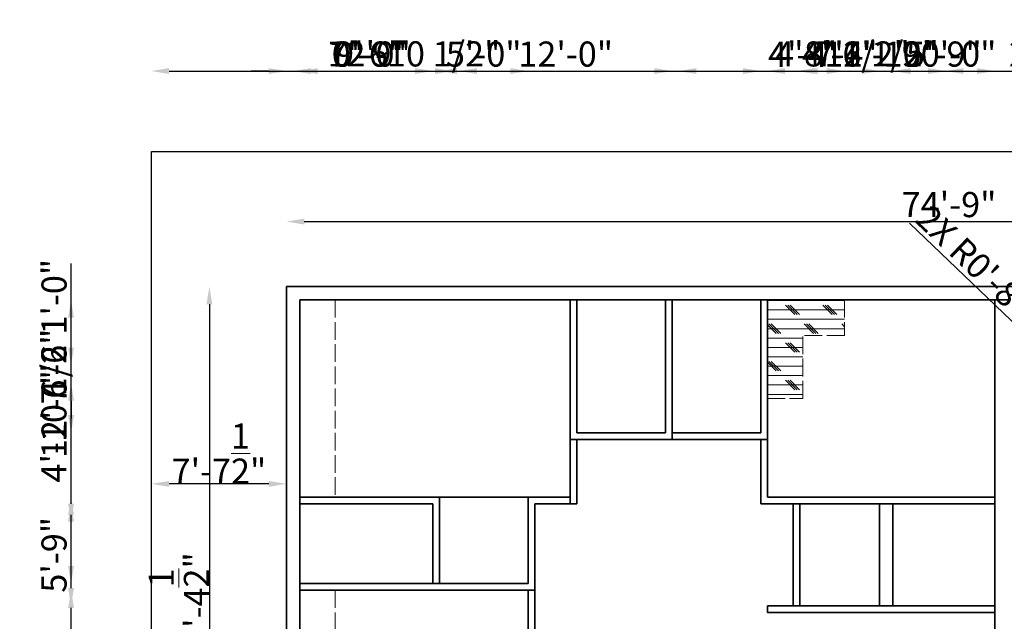
# Model space of a CAD drawing. Units: millimetres. Extents: x 1980 to 3220, y 1535 to 2343.
# Tile 2 of 3: x 1980 to 2647, y 1936 to 2343. Entities that reach past the tile are written whole.
import ezdxf

# ---------------------------------------------------------------- set-up
doc = ezdxf.new("R2010")
doc.units = ezdxf.units.MM
doc.linetypes.add('ACAD_ISO02W100', pattern=[15, 12, -3])
for name, color, linetype, lineweight in [('A-ANNO-DIMS', 2, 'Continuous', 18), ('A-FLOR-FIXT', 9, 'Continuous', 18), ('A-FLOR-FIXT-OVHD', 9, 'ACAD_ISO02W100', 18), ('A-FLOR-FIXT-PATT', 252, 'ACAD_ISO02W100', 13), ('A-WALL', 7, 'Continuous', 35), ('C-PROP', 8, 'Continuous', 25)]:
    doc.layers.add(name, color=color, linetype=linetype, lineweight=lineweight)
doc.styles.get("Standard").update_dxf_attribs({"font": 'arial.ttf'})
doc.dimstyles.new('ISO-25', dxfattribs={"dimtxt": 17, "dimasz": 12, "dimexe": 1.25, "dimexo": 0.625, "dimtad": 1, "dimdec": 1, "dimlunit": 4, "dimtxsty": 'Standard', "dimcen": 2.5, "dimse1": 1, "dimse2": 1, "dimadec": 0, "dimazin": 0, "dimtfac": 1, "dimtdec": 1, "dimtmove": 0, "dimatfit": 3, "dimfxl": 1, "dimarcsym": 0})

# ---------------------------------------------------------------- blocks, each defined once
blk = doc.blocks.new('*D1')
at = {"layer": 'A-ANNO-DIMS', "color": 0, "lineweight": -2, "transparency": 16777216}
blk.add_line((2173.01, 2206.08), (3046.01, 2206.08), dxfattribs=at)
at = {"layer": 'A-ANNO-DIMS', "color": 0, "transparency": 16777216}
for points in [[(2173.01, 2208.08), (2173.01, 2204.08), (2161.01, 2206.08)], [(3046.01, 2208.08), (3046.01, 2204.08), (3058.01, 2206.08)]]:
    blk.add_solid(points, dxfattribs=at)
at = {"layer": 'Defpoints', "color": 0, "transparency": 16777216}
for p in [(3058.01, 2206.08), (2161.01, 2162.1), (3058.01, 2162.1)]:
    blk.add_point(p, dxfattribs=at)
at = {"layer": 'A-ANNO-DIMS', "color": 0, "transparency": 16777216, "insert": (2609.51, 2215.39), "char_height": 17, "attachment_point": 5}
blk.add_mtext('74\'-9"', dxfattribs=at)
blk = doc.blocks.new('*D7')
at = {"layer": 'A-ANNO-DIMS', "color": 0, "lineweight": -2, "transparency": 16777216}
blk.add_line((2149.01, 2028.59), (2081.51, 2028.59), dxfattribs=at)
at = {"layer": 'A-ANNO-DIMS', "color": 0, "transparency": 16777216}
for points in [[(2081.51, 2030.59), (2081.51, 2026.59), (2069.51, 2028.59)], [(2149.01, 2030.59), (2149.01, 2026.59), (2161.01, 2028.59)]]:
    blk.add_solid(points, dxfattribs=at)
at = {"layer": 'Defpoints', "color": 0, "transparency": 16777216}
for p in [(2069.51, 2028.59), (2069.51, 2028.59), (2161.01, 2028.59)]:
    blk.add_point(p, dxfattribs=at)
at = {"layer": 'A-ANNO-DIMS', "color": 0, "transparency": 16777216, "insert": (2115.26, 2049.12), "char_height": 17, "attachment_point": 5}
blk.add_mtext('7\'-7{\\H1x;\\S1/2;}"', dxfattribs=at)
blk = doc.blocks.new('*D8')
at = {"layer": 'A-ANNO-DIMS', "color": 0, "lineweight": -2, "transparency": 16777216}
blk.add_line((2108.81, 2150.1), (2108.81, 1737.6), dxfattribs=at)
at = {"layer": 'A-ANNO-DIMS', "color": 0, "transparency": 16777216}
for points in [[(2106.81, 2150.1), (2110.81, 2150.1), (2108.81, 2162.1)], [(2106.81, 1737.6), (2110.81, 1737.6), (2108.81, 1725.6)]]:
    blk.add_solid(points, dxfattribs=at)
at = {"layer": 'Defpoints', "color": 0, "transparency": 16777216}
for p in [(2161.01, 2162.1), (2108.81, 1725.6), (2161.01, 1725.6)]:
    blk.add_point(p, dxfattribs=at)
at = {"layer": 'A-ANNO-DIMS', "color": 0, "transparency": 16777216, "insert": (2088.13, 1943.85), "char_height": 17, "attachment_point": 5, "rotation": 90}
blk.add_mtext('36\'-4{\\H1x;\\S1/2;}"', dxfattribs=at)
blk = doc.blocks.new('*D9')
at = {"layer": 'A-ANNO-DIMS', "color": 0, "lineweight": -2, "transparency": 16777216}
blk.add_line((2081.51, 2307.95), (3137.51, 2307.95), dxfattribs=at)
at = {"layer": 'A-ANNO-DIMS', "color": 0, "transparency": 16777216}
for points in [[(2081.51, 2309.95), (2081.51, 2305.95), (2069.51, 2307.95)], [(3137.51, 2309.95), (3137.51, 2305.95), (3149.51, 2307.95)]]:
    blk.add_solid(points, dxfattribs=at)
at = {"layer": 'Defpoints', "color": 0, "transparency": 16777216}
for p in [(3149.51, 2307.95), (2069.51, 2253.6), (3149.51, 2253.6)]:
    blk.add_point(p, dxfattribs=at)
at = {"layer": 'A-ANNO-DIMS', "color": 0, "transparency": 16777216, "insert": (2609.51, 2317.25), "char_height": 17, "attachment_point": 5}
blk.add_mtext('90\'-0"', dxfattribs=at)
blk = doc.blocks.new('*D11')
at = {"layer": 'A-ANNO-DIMS', "color": 0, "lineweight": -2, "transparency": 16777216}
blk.add_line((2182.01, 1551.25), (2341.01, 1551.25), dxfattribs=at)
at = {"layer": 'A-ANNO-DIMS', "color": 0, "transparency": 16777216}
for points in [[(2182.01, 1553.25), (2182.01, 1549.25), (2170.01, 1551.25)], [(2341.01, 1553.25), (2341.01, 1549.25), (2353.01, 1551.25)]]:
    blk.add_solid(points, dxfattribs=at)
at = {"layer": 'Defpoints', "color": 0, "transparency": 16777216}
for p in [(2170.01, 2153.1), (2353.01, 2153.1), (2353.01, 1551.25)]:
    blk.add_point(p, dxfattribs=at)
at = {"layer": 'A-ANNO-DIMS', "color": 0, "transparency": 16777216, "insert": (2261.51, 1560.56), "char_height": 17, "attachment_point": 5}
blk.add_mtext('15\'-3"', dxfattribs=at)
blk = doc.blocks.new('*D12')
at = {"layer": 'A-ANNO-DIMS', "color": 0, "lineweight": -2, "transparency": 16777216}
blk.add_line((2369.51, 1551.25), (2405.51, 1551.25), dxfattribs=at)
at = {"layer": 'A-ANNO-DIMS', "color": 0, "transparency": 16777216}
for points in [[(2369.51, 1553.25), (2369.51, 1549.25), (2357.51, 1551.25)], [(2405.51, 1553.25), (2405.51, 1549.25), (2417.51, 1551.25)]]:
    blk.add_solid(points, dxfattribs=at)
at = {"layer": 'Defpoints', "color": 0, "transparency": 16777216}
for p in [(2357.51, 2153.1), (2417.51, 2153.1), (2417.51, 1551.25)]:
    blk.add_point(p, dxfattribs=at)
at = {"layer": 'A-ANNO-DIMS', "color": 0, "transparency": 16777216, "insert": (2387.51, 1560.55), "char_height": 17, "attachment_point": 5}
blk.add_mtext('5\'-0"', dxfattribs=at)
blk = doc.blocks.new('*D13')
at = {"layer": 'A-ANNO-DIMS', "color": 0, "lineweight": -2, "transparency": 16777216}
blk.add_line((2434.01, 1551.25), (2470.01, 1551.25), dxfattribs=at)
at = {"layer": 'A-ANNO-DIMS', "color": 0, "transparency": 16777216}
for points in [[(2434.01, 1553.25), (2434.01, 1549.25), (2422.01, 1551.25)], [(2470.01, 1553.25), (2470.01, 1549.25), (2482.01, 1551.25)]]:
    blk.add_solid(points, dxfattribs=at)
at = {"layer": 'Defpoints', "color": 0, "transparency": 16777216}
for p in [(2422.01, 2153.1), (2482.01, 2153.1), (2482.01, 1551.25)]:
    blk.add_point(p, dxfattribs=at)
at = {"layer": 'A-ANNO-DIMS', "color": 0, "transparency": 16777216, "insert": (2452.01, 1560.55), "char_height": 17, "attachment_point": 5}
blk.add_mtext('5\'-0"', dxfattribs=at)
blk = doc.blocks.new('*D14')
at = {"layer": 'A-ANNO-DIMS', "color": 0, "lineweight": -2, "transparency": 16777216}
blk.add_line((2498.51, 2307.95), (2628.51, 2307.95), dxfattribs=at)
at = {"layer": 'A-ANNO-DIMS', "color": 0, "transparency": 16777216}
for points in [[(2498.51, 2309.95), (2498.51, 2305.95), (2486.51, 2307.95)], [(2628.51, 2309.95), (2628.51, 2305.95), (2640.51, 2307.95)]]:
    blk.add_solid(points, dxfattribs=at)
at = {"layer": 'Defpoints', "color": 0, "transparency": 16777216}
for p in [(2640.51, 2307.95), (2486.51, 2019.6), (2640.51, 2019.6)]:
    blk.add_point(p, dxfattribs=at)
at = {"layer": 'A-ANNO-DIMS', "color": 0, "transparency": 16777216, "insert": (2563.51, 2317.25), "char_height": 17, "attachment_point": 5}
blk.add_mtext('12\'-10"', dxfattribs=at)
blk = doc.blocks.new('*D15')
at = {"layer": 'A-ANNO-DIMS', "color": 0, "lineweight": -2, "transparency": 16777216}
blk.add_line((3203.86, 2031.6), (3203.86, 2141.1), dxfattribs=at)
at = {"layer": 'A-ANNO-DIMS', "color": 0, "transparency": 16777216}
for points in [[(3201.86, 2141.1), (3205.86, 2141.1), (3203.86, 2153.1)], [(3201.86, 2031.6), (3205.86, 2031.6), (3203.86, 2019.6)]]:
    blk.add_solid(points, dxfattribs=at)
at = {"layer": 'Defpoints', "color": 0, "transparency": 16777216}
for p in [(2170.01, 2153.1), (3203.86, 2153.1), (2170.01, 2019.6)]:
    blk.add_point(p, dxfattribs=at)
at = {"layer": 'A-ANNO-DIMS', "color": 0, "transparency": 16777216, "insert": (3194.44, 2086.35), "char_height": 17, "attachment_point": 5, "rotation": 90}
blk.add_mtext('11\'-1 1/2"', dxfattribs=at)
blk = doc.blocks.new('*D16')
at = {"layer": 'A-ANNO-DIMS', "color": 0, "lineweight": -2, "transparency": 16777216}
blk.add_line((3203.86, 2075.1), (3203.86, 2141.1), dxfattribs=at)
at = {"layer": 'A-ANNO-DIMS', "color": 0, "transparency": 16777216}
for points in [[(3201.86, 2141.1), (3205.86, 2141.1), (3203.86, 2153.1)], [(3201.86, 2075.1), (3205.86, 2075.1), (3203.86, 2063.1)]]:
    blk.add_solid(points, dxfattribs=at)
at = {"layer": 'Defpoints', "color": 0, "transparency": 16777216}
for p in [(2357.51, 2153.1), (3203.86, 2153.1), (2357.51, 2063.1)]:
    blk.add_point(p, dxfattribs=at)
at = {"layer": 'A-ANNO-DIMS', "color": 0, "transparency": 16777216, "insert": (3194.55, 2108.1), "char_height": 17, "attachment_point": 5, "rotation": 90}
blk.add_mtext('7\'-6"', dxfattribs=at)
blk = doc.blocks.new('*D17')
at = {"layer": 'A-ANNO-DIMS', "color": 0, "lineweight": -2, "transparency": 16777216}
blk.add_line((2182.01, 2307.95), (2312.51, 2307.95), dxfattribs=at)
at = {"layer": 'A-ANNO-DIMS', "color": 0, "transparency": 16777216}
for points in [[(2182.01, 2309.95), (2182.01, 2305.95), (2170.01, 2307.95)], [(2312.51, 2309.95), (2312.51, 2305.95), (2324.51, 2307.95)]]:
    blk.add_solid(points, dxfattribs=at)
at = {"layer": 'Defpoints', "color": 0, "transparency": 16777216}
for p in [(2324.51, 2307.95), (2170.01, 1830.6), (2324.51, 1830.6)]:
    blk.add_point(p, dxfattribs=at)
at = {"layer": 'A-ANNO-DIMS', "color": 0, "transparency": 16777216, "insert": (2247.26, 2317.36), "char_height": 17, "attachment_point": 5}
blk.add_mtext('12\'-10 1/2"', dxfattribs=at)
blk = doc.blocks.new('*D18')
at = {"layer": 'A-ANNO-DIMS', "color": 0, "lineweight": -2, "transparency": 16777216}
blk.add_line((2015.16, 1842.6), (2015.16, 1944.6), dxfattribs=at)
at = {"layer": 'A-ANNO-DIMS', "color": 0, "transparency": 16777216}
for points in [[(2013.16, 1944.6), (2017.16, 1944.6), (2015.16, 1956.6)], [(2013.16, 1842.6), (2017.16, 1842.6), (2015.16, 1830.6)]]:
    blk.add_solid(points, dxfattribs=at)
at = {"layer": 'Defpoints', "color": 0, "transparency": 16777216}
for p in [(2015.16, 1956.6), (2324.51, 1956.6), (2324.51, 1830.6)]:
    blk.add_point(p, dxfattribs=at)
at = {"layer": 'A-ANNO-DIMS', "color": 0, "transparency": 16777216, "insert": (2005.85, 1893.6), "char_height": 17, "attachment_point": 5, "rotation": 90}
blk.add_mtext('10\'-6"', dxfattribs=at)
blk = doc.blocks.new('*D19')
at = {"layer": 'A-ANNO-DIMS', "color": 0, "lineweight": -2, "transparency": 16777216}
blk.add_line((2182.01, 2307.95), (2248.01, 2307.95), dxfattribs=at)
at = {"layer": 'A-ANNO-DIMS', "color": 0, "transparency": 16777216}
for points in [[(2182.01, 2309.95), (2182.01, 2305.95), (2170.01, 2307.95)], [(2248.01, 2309.95), (2248.01, 2305.95), (2260.01, 2307.95)]]:
    blk.add_solid(points, dxfattribs=at)
at = {"layer": 'Defpoints', "color": 0, "transparency": 16777216}
for p in [(2260.01, 2307.95), (2170.01, 1961.1), (2260.01, 1961.1)]:
    blk.add_point(p, dxfattribs=at)
at = {"layer": 'A-ANNO-DIMS', "color": 0, "transparency": 16777216, "insert": (2215.01, 2317.25), "char_height": 17, "attachment_point": 5}
blk.add_mtext('7\'-6"', dxfattribs=at)
blk = doc.blocks.new('*D20')
at = {"layer": 'A-ANNO-DIMS', "color": 0, "lineweight": -2, "transparency": 16777216}
blk.add_line((2276.51, 2307.95), (2312.51, 2307.95), dxfattribs=at)
at = {"layer": 'A-ANNO-DIMS', "color": 0, "transparency": 16777216}
for points in [[(2276.51, 2309.95), (2276.51, 2305.95), (2264.51, 2307.95)], [(2312.51, 2309.95), (2312.51, 2305.95), (2324.51, 2307.95)]]:
    blk.add_solid(points, dxfattribs=at)
at = {"layer": 'Defpoints', "color": 0, "transparency": 16777216}
for p in [(2324.51, 2307.95), (2264.51, 1961.1), (2324.51, 1961.1)]:
    blk.add_point(p, dxfattribs=at)
at = {"layer": 'A-ANNO-DIMS', "color": 0, "transparency": 16777216, "insert": (2294.51, 2317.25), "char_height": 17, "attachment_point": 5}
blk.add_mtext('5\'-0"', dxfattribs=at)
blk = doc.blocks.new('*D21')
at = {"layer": 'A-ANNO-DIMS', "color": 0, "lineweight": -2, "transparency": 16777216}
for p, q in [((2015.16, 2019.6), (2015.16, 2131.54)), ((2015.16, 1973.1), (2015.16, 2007.6))]:
    blk.add_line(p, q, dxfattribs=at)
at = {"layer": 'A-ANNO-DIMS', "color": 0, "transparency": 16777216}
for points in [[(2013.16, 2007.6), (2017.16, 2007.6), (2015.16, 2019.6)], [(2013.16, 1973.1), (2017.16, 1973.1), (2015.16, 1961.1)]]:
    blk.add_solid(points, dxfattribs=at)
at = {"layer": 'Defpoints', "color": 0, "transparency": 16777216}
for p in [(2015.16, 2019.6), (2324.51, 2019.6), (2324.51, 1961.1)]:
    blk.add_point(p, dxfattribs=at)
at = {"layer": 'A-ANNO-DIMS', "color": 0, "transparency": 16777216, "insert": (2005.74, 2081.57), "char_height": 17, "attachment_point": 5, "rotation": 90}
blk.add_mtext('4\'-10 1/2"', dxfattribs=at)
blk = doc.blocks.new('*D22')
at = {"layer": 'A-ANNO-DIMS', "color": 0, "lineweight": -2, "transparency": 16777216}
blk.add_line((2520.51, 2307.95), (2550.51, 2307.95), dxfattribs=at)
at = {"layer": 'A-ANNO-DIMS', "color": 0, "transparency": 16777216}
for points in [[(2520.51, 2309.95), (2520.51, 2305.95), (2508.51, 2307.95)], [(2550.51, 2309.95), (2550.51, 2305.95), (2562.51, 2307.95)]]:
    blk.add_solid(points, dxfattribs=at)
at = {"layer": 'Defpoints', "color": 0, "transparency": 16777216}
for p in [(2562.51, 2307.95), (2508.51, 1946.1), (2562.51, 1946.1)]:
    blk.add_point(p, dxfattribs=at)
at = {"layer": 'A-ANNO-DIMS', "color": 0, "transparency": 16777216, "insert": (2535.51, 2317.25), "char_height": 17, "attachment_point": 5}
blk.add_mtext('4\'-6"', dxfattribs=at)
blk = doc.blocks.new('*D23')
at = {"layer": 'A-ANNO-DIMS', "color": 0, "lineweight": -2, "transparency": 16777216}
blk.add_line((2583.51, 2307.95), (2628.51, 2307.95), dxfattribs=at)
at = {"layer": 'A-ANNO-DIMS', "color": 0, "transparency": 16777216}
for points in [[(2583.51, 2309.95), (2583.51, 2305.95), (2571.51, 2307.95)], [(2628.51, 2309.95), (2628.51, 2305.95), (2640.51, 2307.95)]]:
    blk.add_solid(points, dxfattribs=at)
at = {"layer": 'Defpoints', "color": 0, "transparency": 16777216}
for p in [(2640.51, 2307.95), (2571.51, 1946.1), (2640.51, 1946.1)]:
    blk.add_point(p, dxfattribs=at)
at = {"layer": 'A-ANNO-DIMS', "color": 0, "transparency": 16777216, "insert": (2606.01, 2317.25), "char_height": 17, "attachment_point": 5}
blk.add_mtext('5\'-9"', dxfattribs=at)
blk = doc.blocks.new('*D24')
at = {"layer": 'A-ANNO-DIMS', "color": 0, "lineweight": -2, "transparency": 16777216}
blk.add_line((2015.16, 1958.1), (2015.16, 2003.1), dxfattribs=at)
at = {"layer": 'A-ANNO-DIMS', "color": 0, "transparency": 16777216}
for points in [[(2013.16, 2003.1), (2017.16, 2003.1), (2015.16, 2015.1)], [(2013.16, 1958.1), (2017.16, 1958.1), (2015.16, 1946.1)]]:
    blk.add_solid(points, dxfattribs=at)
at = {"layer": 'Defpoints', "color": 0, "transparency": 16777216}
for p in [(2015.16, 2015.1), (2640.51, 2015.1), (2640.51, 1946.1)]:
    blk.add_point(p, dxfattribs=at)
at = {"layer": 'A-ANNO-DIMS', "color": 0, "transparency": 16777216, "insert": (2005.85, 1980.6), "char_height": 17, "attachment_point": 5, "rotation": 90}
blk.add_mtext('5\'-9"', dxfattribs=at)
blk = doc.blocks.new('*D25')
at = {"layer": 'A-ANNO-DIMS', "color": 0, "lineweight": -2, "transparency": 16777216}
blk.add_line((2177.51, 2307.95), (2261.51, 2307.95), dxfattribs=at)
at = {"layer": 'A-ANNO-DIMS', "color": 0, "transparency": 16777216}
for points in [[(2177.51, 2309.95), (2177.51, 2305.95), (2165.51, 2307.95)], [(2261.51, 2309.95), (2261.51, 2305.95), (2273.51, 2307.95)]]:
    blk.add_solid(points, dxfattribs=at)
at = {"layer": 'Defpoints', "color": 0, "transparency": 16777216}
for p in [(2273.51, 2307.95), (2165.51, 1734.6), (2273.51, 1734.6)]:
    blk.add_point(p, dxfattribs=at)
at = {"layer": 'A-ANNO-DIMS', "color": 0, "transparency": 16777216, "insert": (2219.51, 2317.25), "char_height": 17, "attachment_point": 5}
blk.add_mtext('9\'-0"', dxfattribs=at)
blk = doc.blocks.new('*D26')
at = {"layer": 'A-ANNO-DIMS', "color": 0, "lineweight": -2, "transparency": 16777216}
blk.add_line((2290.01, 2307.95), (2410.01, 2307.95), dxfattribs=at)
at = {"layer": 'A-ANNO-DIMS', "color": 0, "transparency": 16777216}
for points in [[(2290.01, 2309.95), (2290.01, 2305.95), (2278.01, 2307.95)], [(2410.01, 2309.95), (2410.01, 2305.95), (2422.01, 2307.95)]]:
    blk.add_solid(points, dxfattribs=at)
at = {"layer": 'Defpoints', "color": 0, "transparency": 16777216}
for p in [(2422.01, 2307.95), (2278.01, 1734.6), (2422.01, 1734.6)]:
    blk.add_point(p, dxfattribs=at)
at = {"layer": 'A-ANNO-DIMS', "color": 0, "transparency": 16777216, "insert": (2350.01, 2317.25), "char_height": 17, "attachment_point": 5}
blk.add_mtext('12\'-0"', dxfattribs=at)
blk = doc.blocks.new('*D29')
at = {"layer": 'A-ANNO-DIMS', "color": 0, "lineweight": -2, "transparency": 16777216}
blk.add_line((2518.6, 2307.95), (2595.26, 2307.95), dxfattribs=at)
at = {"layer": 'A-ANNO-DIMS', "color": 0, "transparency": 16777216}
for points in [[(2518.6, 2309.95), (2518.6, 2305.95), (2506.6, 2307.95)], [(2595.26, 2309.95), (2595.26, 2305.95), (2607.26, 2307.95)]]:
    blk.add_solid(points, dxfattribs=at)
at = {"layer": 'Defpoints', "color": 0, "transparency": 16777216}
for p in [(2607.26, 2307.95), (2506.6, 1734.6), (2607.26, 1734.6)]:
    blk.add_point(p, dxfattribs=at)
at = {"layer": 'A-ANNO-DIMS', "color": 0, "transparency": 16777216, "insert": (2556.93, 2317.36), "char_height": 17, "attachment_point": 5}
blk.add_mtext('8\'-4 1/2"', dxfattribs=at)
blk = doc.blocks.new('*D30')
at = {"layer": 'A-ANNO-DIMS', "color": 0, "lineweight": -2, "transparency": 16777216}
for p, q in [((2619.26, 2307.95), (2628.51, 2307.95)), ((2640.51, 2307.95), (2738.85, 2307.95))]:
    blk.add_line(p, q, dxfattribs=at)
at = {"layer": 'A-ANNO-DIMS', "color": 0, "transparency": 16777216}
for points in [[(2619.26, 2309.95), (2619.26, 2305.95), (2607.26, 2307.95)], [(2628.51, 2309.95), (2628.51, 2305.95), (2640.51, 2307.95)]]:
    blk.add_solid(points, dxfattribs=at)
at = {"layer": 'Defpoints', "color": 0, "transparency": 16777216}
for p in [(2640.51, 2307.95), (2607.26, 1734.6), (2640.51, 1734.6)]:
    blk.add_point(p, dxfattribs=at)
at = {"layer": 'A-ANNO-DIMS', "color": 0, "transparency": 16777216, "insert": (2695.68, 2317.36), "char_height": 17, "attachment_point": 5}
blk.add_mtext('2\'-9 1/2"', dxfattribs=at)
blk = doc.blocks.new('*D34')
at = {"layer": 'A-ANNO-DIMS', "color": 0, "lineweight": -2, "transparency": 16777216}
blk.add_line((2015.16, 2015.1), (2015.16, 2141.1), dxfattribs=at)
at = {"layer": 'A-ANNO-DIMS', "color": 0, "transparency": 16777216}
for points in [[(2013.16, 2141.1), (2017.16, 2141.1), (2015.16, 2153.1)], [(2013.16, 2015.1), (2017.16, 2015.1), (2015.16, 2003.1)]]:
    blk.add_solid(points, dxfattribs=at)
at = {"layer": 'Defpoints', "color": 0, "transparency": 16777216}
for p in [(2015.16, 2153.1), (3049.01, 2153.1), (3049.01, 2003.1)]:
    blk.add_point(p, dxfattribs=at)
at = {"layer": 'A-ANNO-DIMS', "color": 0, "transparency": 16777216, "insert": (2005.85, 2078.1), "char_height": 17, "attachment_point": 5, "rotation": 90}
blk.add_mtext('12\'-6"', dxfattribs=at)
blk = doc.blocks.new('*D35')
at = {"layer": 'A-ANNO-DIMS', "color": 0, "lineweight": -2, "transparency": 16777216}
blk.add_line((2015.16, 2075.1), (2015.16, 2141.1), dxfattribs=at)
at = {"layer": 'A-ANNO-DIMS', "color": 0, "transparency": 16777216}
for points in [[(2013.16, 2141.1), (2017.16, 2141.1), (2015.16, 2153.1)], [(2013.16, 2075.1), (2017.16, 2075.1), (2015.16, 2063.1)]]:
    blk.add_solid(points, dxfattribs=at)
at = {"layer": 'Defpoints', "color": 0, "transparency": 16777216}
for p in [(2015.16, 2153.1), (2923.51, 2153.1), (2923.51, 2063.1)]:
    blk.add_point(p, dxfattribs=at)
at = {"layer": 'A-ANNO-DIMS', "color": 0, "transparency": 16777216, "insert": (2005.85, 2108.1), "char_height": 17, "attachment_point": 5, "rotation": 90}
blk.add_mtext('7\'-6"', dxfattribs=at)
blk = doc.blocks.new('*D48')
at = {"layer": 'A-ANNO-DIMS', "color": 0, "lineweight": -2, "transparency": 16777216}
for p, q in [((2015.16, 2120.82), (2015.16, 2177.66)), ((2015.16, 2096.82), (2015.16, 2108.82)), ((2015.16, 2084.82), (2015.16, 2072.82))]:
    blk.add_line(p, q, dxfattribs=at)
at = {"layer": 'A-ANNO-DIMS', "color": 0, "transparency": 16777216}
for points in [[(2013.16, 2120.82), (2017.16, 2120.82), (2015.16, 2108.82)], [(2013.16, 2084.82), (2017.16, 2084.82), (2015.16, 2096.82)]]:
    blk.add_solid(points, dxfattribs=at)
at = {"layer": 'Defpoints', "color": 0, "transparency": 16777216}
for p in [(2015.16, 2108.82), (2649.51, 2108.82), (2649.51, 2096.82)]:
    blk.add_point(p, dxfattribs=at)
at = {"layer": 'A-ANNO-DIMS', "color": 0, "transparency": 16777216, "insert": (2005.85, 2155.24), "char_height": 17, "attachment_point": 5, "rotation": 90}
blk.add_mtext('1\'-0"', dxfattribs=at)
blk = doc.blocks.new('*D49')
at = {"layer": 'A-ANNO-DIMS', "color": 0, "lineweight": -2, "transparency": 16777216}
for p, q in [((2149.01, 2307.95), (2137.01, 2307.95)), ((2161.01, 2307.95), (2170.01, 2307.95)), ((2182.01, 2307.95), (2240.45, 2307.95))]:
    blk.add_line(p, q, dxfattribs=at)
at = {"layer": 'A-ANNO-DIMS', "color": 0, "transparency": 16777216}
for points in [[(2149.01, 2309.95), (2149.01, 2305.95), (2161.01, 2307.95)], [(2182.01, 2309.95), (2182.01, 2305.95), (2170.01, 2307.95)]]:
    blk.add_solid(points, dxfattribs=at)
at = {"layer": 'Defpoints', "color": 0, "transparency": 16777216}
for p in [(2170.01, 2307.95), (2161.01, 2162.1), (2170.01, 2153.1)]:
    blk.add_point(p, dxfattribs=at)
at = {"layer": 'A-ANNO-DIMS', "color": 0, "transparency": 16777216, "insert": (2217.23, 2317.25), "char_height": 17, "attachment_point": 5}
blk.add_mtext('0\'-9"', dxfattribs=at)
blk = doc.blocks.new('*D50')
at = {"layer": 'A-ANNO-DIMS', "color": 0, "lineweight": -2, "transparency": 16777216}
for p, q in [((2405.51, 1551.25), (2393.51, 1551.25)), ((2417.51, 1551.25), (2422.01, 1551.25)), ((2434.01, 1551.25), (2532.06, 1551.25))]:
    blk.add_line(p, q, dxfattribs=at)
at = {"layer": 'A-ANNO-DIMS', "color": 0, "transparency": 16777216}
for points in [[(2405.51, 1553.25), (2405.51, 1549.25), (2417.51, 1551.25)], [(2434.01, 1553.25), (2434.01, 1549.25), (2422.01, 1551.25)]]:
    blk.add_solid(points, dxfattribs=at)
at = {"layer": 'Defpoints', "color": 0, "transparency": 16777216}
for p in [(2417.51, 2063.1), (2422.01, 2063.1), (2422.01, 1551.25)]:
    blk.add_point(p, dxfattribs=at)
at = {"layer": 'A-ANNO-DIMS', "color": 0, "transparency": 16777216, "insert": (2489.03, 1560.66), "char_height": 17, "attachment_point": 5}
blk.add_mtext('0\'-4 1/2"', dxfattribs=at)
blk = doc.blocks.new('*D51')
at = {"layer": 'A-ANNO-DIMS', "color": 0, "lineweight": -2, "transparency": 16777216}
blk.add_line((2498.508481, 2307.945639), (2526.687065, 2307.945639), dxfattribs=at)
at = {"layer": 'A-ANNO-DIMS', "color": 0, "transparency": 16777216}
for points in [[(2498.508481, 2309.945639), (2498.508481, 2305.945639), (2486.508481, 2307.945639)], [(2526.687065, 2309.945639), (2526.687065, 2305.945639), (2538.687065, 2307.945639)]]:
    blk.add_solid(points, dxfattribs=at)
at = {"layer": 'Defpoints', "color": 0, "transparency": 16777216}
for p in [(2538.687065, 2307.945639), (2486.508481, 2153.095639), (2538.687065, 2153.095639)]:
    blk.add_point(p, dxfattribs=at)
at = {"layer": 'A-ANNO-DIMS', "color": 0, "transparency": 16777216, "insert": (2512.597773, 2317.070639), "char_height": 17, "attachment_point": 5}
blk.add_mtext('4\'-4"', dxfattribs=at)
blk = doc.blocks.new('*D52')
at = {"layer": 'A-ANNO-DIMS', "color": 0, "lineweight": -2, "transparency": 16777216}
blk.add_line((3203.86, 2098.35), (3203.86, 2141.1), dxfattribs=at)
at = {"layer": 'A-ANNO-DIMS', "color": 0, "transparency": 16777216}
for points in [[(3201.86, 2141.1), (3205.86, 2141.1), (3203.86, 2153.1)], [(3201.86, 2098.35), (3205.86, 2098.35), (3203.86, 2086.35)]]:
    blk.add_solid(points, dxfattribs=at)
at = {"layer": 'Defpoints', "color": 0, "transparency": 16777216}
for p in [(2538.69, 2153.1), (3203.86, 2153.1), (2510.51, 2086.35)]:
    blk.add_point(p, dxfattribs=at)
at = {"layer": 'A-ANNO-DIMS', "color": 0, "transparency": 16777216, "insert": (3194.59, 2119.72), "char_height": 17, "attachment_point": 5, "rotation": 90}
blk.add_mtext('5\'-7"', dxfattribs=at)
blk = doc.blocks.new('*D53')
at = {"layer": 'A-ANNO-DIMS', "color": 0, "lineweight": -2, "transparency": 16777216}
for p, q in [((2474.51, 1551.25), (2462.51, 1551.25)), ((2486.51, 1551.25), (2510.51, 1551.25)), ((2522.51, 1551.25), (2581.24, 1551.25))]:
    blk.add_line(p, q, dxfattribs=at)
at = {"layer": 'A-ANNO-DIMS', "color": 0, "transparency": 16777216}
for points in [[(2474.51, 1553.25), (2474.51, 1549.25), (2486.51, 1551.25)], [(2522.51, 1553.25), (2522.51, 1549.25), (2510.51, 1551.25)]]:
    blk.add_solid(points, dxfattribs=at)
at = {"layer": 'Defpoints', "color": 0, "transparency": 16777216}
for p in [(2486.51, 2086.35), (2510.51, 2086.35), (2510.51, 1551.25)]:
    blk.add_point(p, dxfattribs=at)
at = {"layer": 'A-ANNO-DIMS', "color": 0, "transparency": 16777216, "insert": (2557.87, 1560.55), "char_height": 17, "attachment_point": 5}
blk.add_mtext('2\'-0"', dxfattribs=at)
blk = doc.blocks.new('*D54')
at = {"layer": 'A-ANNO-DIMS', "color": 0, "lineweight": -2, "transparency": 16777216}
for p, q in [((2438.51, 2307.95), (2470.01, 2307.95)), ((2482.01, 2307.95), (2580.75, 2307.95))]:
    blk.add_line(p, q, dxfattribs=at)
at = {"layer": 'A-ANNO-DIMS', "color": 0, "transparency": 16777216}
for points in [[(2438.51, 2309.95), (2438.51, 2305.95), (2426.51, 2307.95)], [(2470.01, 2309.95), (2470.01, 2305.95), (2482.01, 2307.95)]]:
    blk.add_solid(points, dxfattribs=at)
at = {"layer": 'Defpoints', "color": 0, "transparency": 16777216}
for p in [(2482.01, 2307.95), (2426.51, 1799.1), (2482.01, 1799.1)]:
    blk.add_point(p, dxfattribs=at)
at = {"layer": 'A-ANNO-DIMS', "color": 0, "transparency": 16777216, "insert": (2537.38, 2317.36), "char_height": 17, "attachment_point": 5}
blk.add_mtext('4\'-7 1/2"', dxfattribs=at)
blk = doc.blocks.new('*D57')
at = {"layer": 'A-ANNO-DIMS', "color": 0, "lineweight": -2, "transparency": 16777216}
for p, q in [((2550.51, 1551.25), (2538.51, 1551.25)), ((2562.51, 1551.25), (2571.51, 1551.25)), ((2583.51, 1551.25), (2641.95, 1551.25))]:
    blk.add_line(p, q, dxfattribs=at)
at = {"layer": 'A-ANNO-DIMS', "color": 0, "transparency": 16777216}
for points in [[(2550.51, 1553.25), (2550.51, 1549.25), (2562.51, 1551.25)], [(2583.51, 1553.25), (2583.51, 1549.25), (2571.51, 1551.25)]]:
    blk.add_solid(points, dxfattribs=at)
at = {"layer": 'Defpoints', "color": 0, "transparency": 16777216}
for p in [(2562.51, 1946.1), (2571.51, 1946.1), (2571.51, 1551.25)]:
    blk.add_point(p, dxfattribs=at)
at = {"layer": 'A-ANNO-DIMS', "color": 0, "transparency": 16777216, "insert": (2618.73, 1560.55), "char_height": 17, "attachment_point": 5}
blk.add_mtext('0\'-9"', dxfattribs=at)
blk = doc.blocks.new('*D58')
at = {"layer": 'A-ANNO-DIMS', "color": 0, "lineweight": -2, "transparency": 16777216}
for p, q in [((2582.78, 2205.03), (2663.33, 2127.9)), ((2677.78, 2114.07), (2672, 2119.6))]:
    blk.add_line(p, q, dxfattribs=at)
at = {"layer": 'A-ANNO-DIMS', "color": 0, "transparency": 16777216}
blk.add_solid([(2664.72, 2129.34), (2661.95, 2126.45), (2672, 2119.6)], dxfattribs=at)
at = {"layer": 'Defpoints', "color": 0, "transparency": 16777216}
for p in [(2672, 2119.6), (2677.78, 2114.07)]:
    blk.add_point(p, dxfattribs=at)
at = {"layer": 'A-ANNO-DIMS', "color": 0, "transparency": 16777216, "insert": (2625.16, 2177.34), "char_height": 17, "attachment_point": 5, "rotation": 316.24382}
blk.add_mtext('2X R0\'-8"', dxfattribs=at)

msp = doc.modelspace()

# ---------------------------------------------------------------- hatches: boundary and pattern name
at = {"layer": 'A-FLOR-FIXT-PATT'}
h = msp.add_hatch(dxfattribs=at)
h.set_pattern_fill('CORK', color=256, scale=2)
h.set_pattern_definition([(0, (0, 0), (0, 6.35), []), (135, (3.175, -3.175), (-12.70001, -12.70001), [8.98026, -8.98026]), (135, (4.763, -3.175), (-12.70001, -12.70001), [8.98026, -8.98026]), (135, (6.35, -3.175), (-12.70001, -12.70001), [8.98026, -8.98026])])
h.paths.add_polyline_path([(2510.51, 2129.1), (2538.69, 2129.1), (2538.69, 2153.1), (2486.51, 2153.1), (2486.51, 2086.35), (2510.51, 2086.35)])

# ---------------------------------------------------------------- linework, layer by layer
at = {"layer": 'A-FLOR-FIXT'}
for p, q in [((2170.01, 2153.1), (2200.01, 2153.1)), ((2170.01, 2153.1), (2194.01, 2153.1)), ((2486.51, 2153.1), (2532.27, 2153.1))]:
    msp.add_line(p, q, dxfattribs=at)
at = {"layer": 'A-FLOR-FIXT-OVHD'}
for p, q in [((2194.01, 2153.1), (2194.01, 2019.6)), ((2538.69, 2153.1), (2538.69, 2129.1)), ((2538.69, 2129.1), (2510.51, 2129.1)), ((2510.51, 2086.35), (2510.51, 2129.1)), ((2486.51, 2086.35), (2510.51, 2086.35)), ((2194.01, 1956.6), (2194.01, 1830.6))]:
    msp.add_line(p, q, dxfattribs=at)
at = {"layer": 'A-WALL'}
for p, q in [((2161.01, 1725.6), (2161.01, 2162.1)), ((2161.01, 2162.1), (3058.01, 2162.1)), ((2170.01, 1830.6), (2170.01, 2153.1)), ((2170.01, 2153.1), (2649.51, 2153.1)), ((2353.01, 2015.1), (2353.01, 2153.1)), ((2357.51, 2063.1), (2357.51, 2153.1)), ((2417.51, 2063.1), (2417.51, 2153.1)), ((2422.01, 2058.6), (2422.01, 2153.1)), ((2482.01, 2063.1), (2482.01, 2153.1)), ((2486.51, 2019.6), (2486.51, 2153.1)), ((2640.51, 1734.6), (2640.51, 2153.1)), ((2357.51, 2063.1), (2417.51, 2063.1)), ((2422.01, 2063.1), (2482.01, 2063.1)), ((2353.01, 2058.6), (2486.51, 2058.6)), ((2357.51, 2015.1), (2357.51, 2058.6)), ((2482.01, 2015.1), (2482.01, 2058.6)), ((2170.01, 2019.6), (2353.01, 2019.6)), ((2170.01, 2015.1), (2260.01, 2015.1)), ((2260.01, 1961.1), (2260.01, 2015.1)), ((2264.51, 1961.1), (2264.51, 2019.6)), ((2324.51, 1961.1), (2324.51, 2019.6)), ((2329.01, 1956.6), (2329.01, 2015.1)), ((2329.01, 2015.1), (2357.51, 2015.1)), ((2482.01, 2015.1), (2640.51, 2015.1)), ((2486.51, 2019.6), (2640.51, 2019.6)), ((2504.01, 1946.1), (2504.01, 2015.1)), ((2508.51, 1946.1), (2508.51, 2015.1)), ((2562.51, 1946.1), (2562.51, 2015.1)), ((2571.51, 1946.1), (2571.51, 2015.1)), ((2170.01, 1961.1), (2264.51, 1961.1)), ((2264.51, 1961.1), (2324.51, 1961.1)), ((2170.01, 1956.6), (2329.01, 1956.6)), ((2324.51, 1956.6), (2324.51, 1830.6)), ((2329.01, 1956.6), (2329.01, 1826.1)), ((2486.51, 1946.1), (2640.51, 1946.1)), ((2486.51, 1941.6), (2486.51, 1946.1)), ((2486.51, 1941.6), (2640.51, 1941.6))]:
    msp.add_line(p, q, dxfattribs=at)
at = {"layer": 'C-PROP'}
msp.add_lwpolyline([(2069.51, 2253.6), (3149.51, 2253.6), (3149.51, 1605.6), (2069.51, 1605.6)], close=True, dxfattribs=at)

# ---------------------------------------------------------------- dimensions: what is measured, and where the dimension line sits
at = {"layer": 'A-ANNO-DIMS'}
for base, p1, p2, override, picture, middle in [((2324.51, 2307.95), (2170.01, 1830.6), (2324.51, 1830.6), {"dimdec": 1, "dimlfac": 1, "dimrnd": 0, "dimzin": 1, "dimdsep": 46, "dimlunit": 4, "dimfrac": 2}, '*D17', (2247.26, 2317.36)), ((2482.01, 2307.95), (2426.51, 1799.1), (2482.01, 1799.1), {"dimdec": 1, "dimlfac": 1, "dimrnd": 0, "dimzin": 1, "dimdsep": 46, "dimlunit": 4, "dimfrac": 2}, '*D54', (2537.38, 2317.36)), ((2607.26, 2307.95), (2506.6, 1734.6), (2607.26, 1734.6), {"dimdec": 1, "dimlfac": 1, "dimrnd": 0, "dimzin": 1, "dimdsep": 46, "dimlunit": 4, "dimfrac": 2}, '*D29', (2556.93, 2317.36)), ((2640.508481, 2307.945639), (2607.258481, 1734.595639), (2640.508481, 1734.595639), {"dimdec": 1, "dimlfac": 1, "dimrnd": 0, "dimzin": 1, "dimdsep": 46, "dimlunit": 4, "dimfrac": 2}, '*D30', (2695.67986572, 2317.3605435)), ((3149.51, 2307.95), (2069.51, 2253.6), (3149.51, 2253.6), {"dimdec": 1, "dimlfac": 1, "dimrnd": 0, "dimzin": 1, "dimdsep": 46, "dimlunit": 4, "dimfrac": 2}, '*D9', (2609.51, 2317.25)), ((2170.01, 2307.95), (2161.01, 2162.1), (2170.01, 2153.1), {"dimdec": 1, "dimlfac": 1, "dimrnd": 0, "dimzin": 1, "dimdsep": 46, "dimlunit": 4, "dimfrac": 2}, '*D49', (2217.23, 2317.25)), ((2273.51, 2307.95), (2165.51, 1734.6), (2273.51, 1734.6), {"dimdec": 1, "dimlfac": 1, "dimrnd": 0, "dimzin": 1, "dimdsep": 46, "dimlunit": 4, "dimfrac": 2}, '*D25', (2219.51, 2317.25)), ((2260.01, 2307.95), (2170.01, 1961.1), (2260.01, 1961.1), {"dimdec": 1, "dimlfac": 1, "dimrnd": 0, "dimzin": 1, "dimdsep": 46, "dimlunit": 4, "dimfrac": 2}, '*D19', (2215.01, 2317.25)), ((2324.51, 2307.95), (2264.51, 1961.1), (2324.51, 1961.1), {"dimdec": 1, "dimlfac": 1, "dimrnd": 0, "dimzin": 1, "dimdsep": 46, "dimlunit": 4, "dimfrac": 2}, '*D20', (2294.51, 2317.25)), ((2422.01, 2307.95), (2278.01, 1734.6), (2422.01, 1734.6), {"dimdec": 1, "dimlfac": 1, "dimrnd": 0, "dimzin": 1, "dimdsep": 46, "dimlunit": 4, "dimfrac": 2}, '*D26', (2350.01, 2317.25)), ((2640.51, 2307.95), (2486.51, 2019.6), (2640.51, 2019.6), {"dimdec": 1, "dimlfac": 1, "dimrnd": 0, "dimzin": 1, "dimdsep": 46, "dimlunit": 4, "dimfrac": 2}, '*D14', (2563.51, 2317.25)), ((2538.69, 2307.95), (2486.51, 2153.1), (2538.69, 2153.1), {"dimdec": 1, "dimlfac": 1, "dimrnd": 0, "dimzin": 1, "dimdsep": 46, "dimlunit": 4, "dimfrac": 2}, '*D51', (2512.6, 2317.07)), ((2562.51, 2307.95), (2508.51, 1946.1), (2562.51, 1946.1), {"dimdec": 1, "dimlfac": 1, "dimrnd": 0, "dimzin": 1, "dimdsep": 46, "dimlunit": 4, "dimfrac": 2}, '*D22', (2535.51, 2317.25)), ((2640.51, 2307.95), (2571.51, 1946.1), (2640.51, 1946.1), {"dimdec": 1, "dimlfac": 1, "dimrnd": 0, "dimzin": 1, "dimdsep": 46, "dimlunit": 4, "dimfrac": 2}, '*D23', (2606.01, 2317.25)), ((3058.01, 2206.08), (2161.01, 2162.1), (3058.01, 2162.1), {"dimclrd": 0, "dimclre": 0, "dimclrt": 0}, '*D1', (2609.51, 2215.39)), ((2353.01, 1551.25), (2170.01, 2153.1), (2353.01, 2153.1), {"dimdec": 1, "dimlfac": 1, "dimrnd": 0, "dimzin": 1, "dimdsep": 46, "dimlunit": 4, "dimfrac": 2}, '*D11', (2261.51, 1560.56)), ((2417.51, 1551.25), (2357.51, 2153.1), (2417.51, 2153.1), {"dimdec": 1, "dimlfac": 1, "dimrnd": 0, "dimzin": 1, "dimdsep": 46, "dimlunit": 4, "dimfrac": 2}, '*D12', (2387.51, 1560.55)), ((2482.01, 1551.25), (2422.01, 2153.1), (2482.01, 2153.1), {"dimdec": 1, "dimlfac": 1, "dimrnd": 0, "dimzin": 1, "dimdsep": 46, "dimlunit": 4, "dimfrac": 2}, '*D13', (2452.01, 1560.55)), ((2510.51, 1551.25), (2486.51, 2086.35), (2510.51, 2086.35), {"dimdec": 1, "dimlfac": 1, "dimrnd": 0, "dimzin": 1, "dimdsep": 46, "dimlunit": 4, "dimfrac": 2}, '*D53', (2557.87, 1560.55)), ((2069.51, 2028.59), (2161.01, 2028.59), (2069.51, 2028.59), {"dimclrd": 0, "dimclre": 0, "dimclrt": 0}, '*D7', (2115.26, 2049.12)), ((2422.01, 1551.25), (2417.51, 2063.1), (2422.01, 2063.1), {"dimdec": 1, "dimlfac": 1, "dimrnd": 0, "dimzin": 1, "dimdsep": 46, "dimlunit": 4, "dimfrac": 2}, '*D50', (2489.03, 1560.66)), ((2571.51, 1551.25), (2562.51, 1946.1), (2571.51, 1946.1), {"dimdec": 1, "dimlfac": 1, "dimrnd": 0, "dimzin": 1, "dimdsep": 46, "dimlunit": 4, "dimfrac": 2}, '*D57', (2618.73, 1560.55))]:
    dim = msp.add_linear_dim(base=base, p1=p1, p2=p2, dimstyle='ISO-25', override=override, dxfattribs=at)
    dim.commit()
    dim.dimension.update_dxf_attribs({"geometry": picture, "text_midpoint": middle})
dim = msp.add_radius_dim(center=(2677.78, 2114.07), mpoint=(2672, 2119.6), text='2X <>', dimstyle='ISO-25', override={"dimdec": 1, "dimlfac": 1, "dimrnd": 0, "dimzin": 1, "dimdsep": 46, "dimlunit": 4, "dimfrac": 2}, dxfattribs=at)
dim.commit()
dim.dimension.update_dxf_attribs({"geometry": '*D58', "text_midpoint": (2625.16, 2177.34)})
for base, p1, p2, override, picture, middle in [((2015.16, 2108.82), (2649.51, 2096.82), (2649.51, 2108.82), {"dimdec": 1, "dimlfac": 1, "dimrnd": 0, "dimzin": 1, "dimdsep": 46, "dimlunit": 4, "dimfrac": 2}, '*D48', (2005.85, 2155.24)), ((2108.81, 1725.6), (2161.01, 2162.1), (2161.01, 1725.6), {"dimclrd": 0, "dimclre": 0, "dimclrt": 0}, '*D8', (2088.13, 1943.85)), ((2015.16, 2153.1), (3049.01, 2003.1), (3049.01, 2153.1), {"dimdec": 1, "dimlfac": 1, "dimrnd": 0, "dimzin": 1, "dimdsep": 46, "dimlunit": 4, "dimfrac": 2}, '*D34', (2005.85, 2078.1)), ((2015.16, 2153.1), (2923.51, 2063.1), (2923.51, 2153.1), {"dimdec": 1, "dimlfac": 1, "dimrnd": 0, "dimzin": 1, "dimdsep": 46, "dimlunit": 4, "dimfrac": 2}, '*D35', (2005.85, 2108.1)), ((3203.86, 2153.1), (2170.01, 2019.6), (2170.01, 2153.1), {"dimdec": 1, "dimlfac": 1, "dimrnd": 0, "dimzin": 1, "dimdsep": 46, "dimlunit": 4, "dimfrac": 2}, '*D15', (3194.44, 2086.35)), ((3203.86, 2153.1), (2357.51, 2063.1), (2357.51, 2153.1), {"dimdec": 1, "dimlfac": 1, "dimrnd": 0, "dimzin": 1, "dimdsep": 46, "dimlunit": 4, "dimfrac": 2}, '*D16', (3194.55, 2108.1)), ((3203.858481, 2153.095639), (2510.508481, 2086.345639), (2538.687065, 2153.095639), {"dimdec": 1, "dimlfac": 1, "dimrnd": 0, "dimzin": 1, "dimdsep": 46, "dimlunit": 4, "dimfrac": 2}, '*D52', (3194.58852875, 2119.720639)), ((2015.16, 2019.6), (2324.51, 1961.1), (2324.51, 2019.6), {"dimdec": 1, "dimlfac": 1, "dimrnd": 0, "dimzin": 1, "dimdsep": 46, "dimlunit": 4, "dimfrac": 2}, '*D21', (2005.74, 2081.57)), ((2015.16, 2015.1), (2640.51, 1946.1), (2640.51, 2015.1), {"dimdec": 1, "dimlfac": 1, "dimrnd": 0, "dimzin": 1, "dimdsep": 46, "dimlunit": 4, "dimfrac": 2}, '*D24', (2005.85, 1980.6)), ((2015.16, 1956.6), (2324.51, 1830.6), (2324.51, 1956.6), {"dimdec": 1, "dimlfac": 1, "dimrnd": 0, "dimzin": 1, "dimdsep": 46, "dimlunit": 4, "dimfrac": 2}, '*D18', (2005.85, 1893.6))]:
    dim = msp.add_linear_dim(base=base, p1=p1, p2=p2, angle=90, dimstyle='ISO-25', override=override, dxfattribs=at)
    dim.commit()
    dim.dimension.update_dxf_attribs({"geometry": picture, "text_midpoint": middle})

doc.saveas('drawing.dxf')
